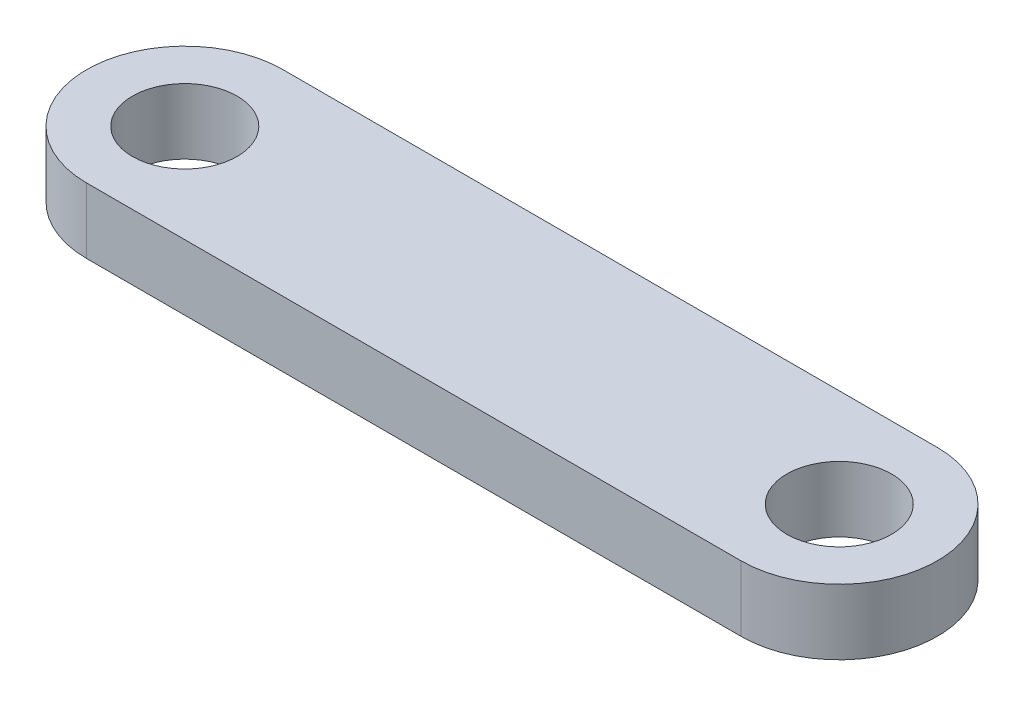
from build123d import *

# Parameters (mm, degrees)
LINK_PLATE_DEPTH     = 2.5
PIN_HOLES_SKETCH_R   = 4
PIN_HOLES_2X_8_DEPTH = 2.5


with BuildPart() as part:
    # Link Profile Sketch → Link Plate (new, symmetric)
    with BuildSketch(Plane(origin=(0, 0, 0), x_dir=(1, 0, 0), z_dir=(0, 1, 0))):
        with BuildLine():
            Line((-25, 7.5), (25, 7.5))
            ThreePointArc((25, 7.5), (32.5, 0), (25, -7.5))
            Line((25, -7.5), (-25, -7.5))
            ThreePointArc((-25, -7.5), (-32.5, 0), (-25, 7.5))
        make_face()
    extrude(amount=LINK_PLATE_DEPTH, both=True)

    # Pin Holes Sketch → Pin Holes 2xØ8 (cut, symmetric)
    with BuildSketch(Plane(origin=(0, 0, 0), x_dir=(1, 0, 0), z_dir=(0, 1, 0))):
        with Locations(Location((-25, 0, 0), (0, 0, 270))):
            Circle(PIN_HOLES_SKETCH_R)
        with Locations(Location((25, 0, 0), (0, 0, 270))):
            Circle(PIN_HOLES_SKETCH_R)
    extrude(amount=PIN_HOLES_2X_8_DEPTH, both=True, mode=Mode.SUBTRACT)


solid = part.part
